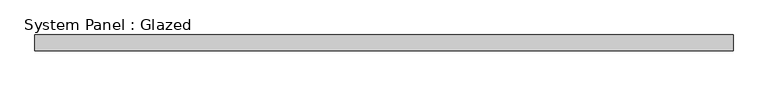
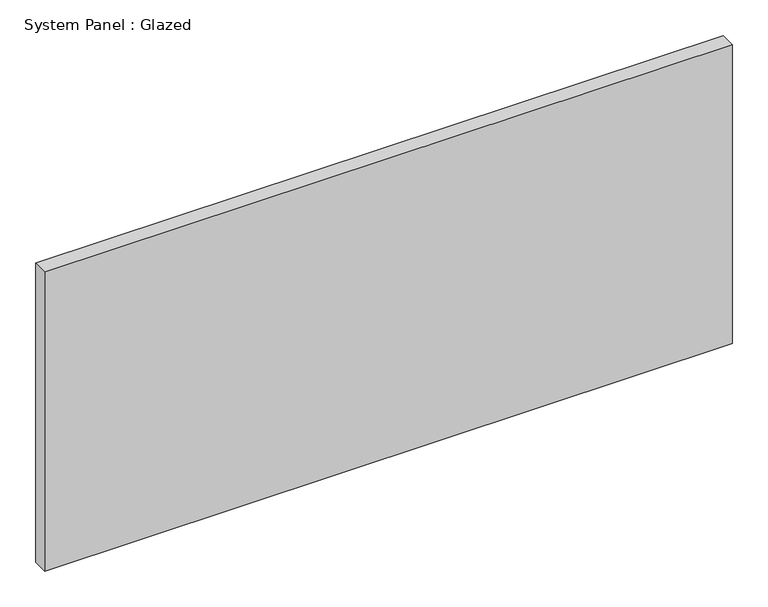
"""IFC4 building model written with IfcOpenShell, lengths in millimetres: plate geometry, System Panel : Glazed."""

from ifc_helpers import new_model, si_unit, origin, origin_with_axes, place, context, project, spatial, polyline, outline, extrude, source, transform, mapped, element, save


def system_panel_glazed_b788c8e7(model_context):
    return source(origin(), model_context, "Body", "SweptSolid", [
        extrude(outline(polyline([(558.7999999, 19.05), (-558.7999999, 19.05), (-558.7999999, 44.45), (558.7999999, 44.45), (558.7999999, 19.05)])), origin_with_axes(), (0.0, 0.0, 1.0), 514.35),
    ])


if __name__ == "__main__":
    model = new_model("IFC4")
    model_context = context("Model", 3, world=origin())
    ifc_project = project(units=[si_unit("LENGTHUNIT", "METRE", prefix="MILLI")], contexts=[model_context])
    site = spatial("IfcSite", under=ifc_project)
    building = spatial("IfcBuilding", under=site)
    placement = place(None, origin())
    system_panel_glazed_shape = system_panel_glazed_b788c8e7(model_context)
    element("IfcPlate", 1, ObjectType="System Panel : Glazed", at=placement, inside=building, context=model_context, shape_type="MappedRepresentation", body=[
        mapped(system_panel_glazed_shape, transform((0.0, 0.0, 0.0), x_axis=(1.0, 0.0, 0.0), y_axis=(0.0, 1.0, 0.0), z_axis=(0.0, 0.0, 1.0))),
    ])
    save(model, "model.ifc")

# Revit data of these elements
# Type "System Panel : Glazed"
#   Construction Type Id = "GSP4R"
#   Analytic Construction = "1/8 in Pilkington single glazing"
#   Visual Light Transmittance = 0.9
#   Solar Heat Gain Coefficient = 0.86
#   Heat Transfer Coefficient (U) = 1.18115 BTU/(h·ft²·°F)
#   Define Thermal Properties by = 1
# Element 1 (IfcPlate, "System Panel : Glazed")
#   Materials on its faces: "Glass"
# Materials
#   "Glass": class "Glass", colour RGB 0 128 192, transparency 0.75, Description = "Soda Lime Glass", Cost = 0
